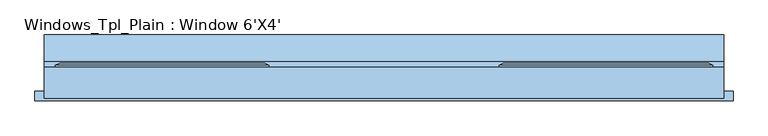
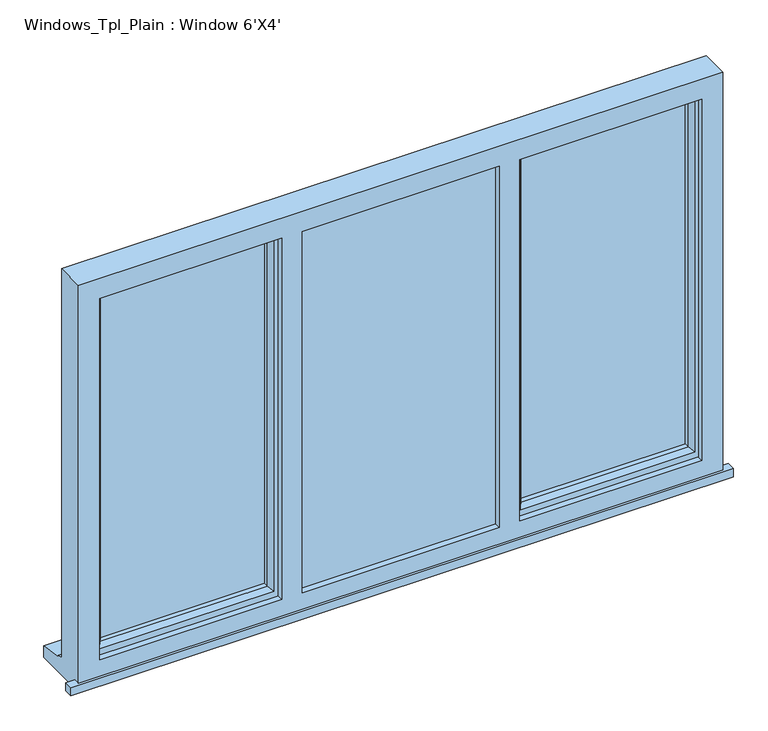
"""IFC4 building model written with IfcOpenShell, lengths in millimetres: window geometry, Windows_Tpl_Plain : Window 6'X4'."""

from ifc_helpers import new_model, si_unit, frame, origin, place, context, project, spatial, polyline, outline, extrude, faceted_brep, source, transform, mapped, element, save


def windows_tpl_plain_window_6_x4_c470b90d(model_context):
    return source(origin(), model_context, "Body", "SolidModel", [
        extrude(outline(polyline([(-1519.2, -73.6934322), (-1519.2, -48.6934322), (-1494.2, -48.6934322), (-1494.2, -67.3934322), (334.6, -67.3934322), (334.6, -48.6934322), (359.6, -48.6934322), (359.6, -73.6934322), (-1519.2, -73.6934322)])), frame((0.0, 0.0, 890.8), z_axis=(0.0, 0.0, 1.0), x_axis=(1.0, 0.0, 0.0)), (0.0, 0.0, 1.0), 25.0),
        faceted_brep([(-270.0, 15.6065678, 2080.0), (-270.0, 21.3800705, 2080.0), (-270.0, 21.3800705, 943.8), (-270.0, 15.6065678, 943.8), (-260.0, -49.3934322, 2070.0), (-260.0, 15.6065678, 2070.0), (-260.0, 15.6065678, 953.8), (-260.0, -49.3934322, 953.8), (-220.0, -34.9005323, 2030.0), (-230.1480377, -49.3934322, 2040.1480377), (-230.1480377, -49.3934322, 983.6519623), (-220.0, -34.9005323, 993.8), (-220.0, -20.3934322, 2030.0), (-220.0, -20.3934322, 993.8), (-230.0, 3.6065678, 2040.0), (-230.0, -20.3934322, 2040.0), (-230.0, -20.3934322, 983.8), (-230.0, 3.6065678, 983.8), (-220.0, 21.3800705, 2030.0), (-220.0, 3.6065678, 2030.0), (-220.0, 3.6065678, 993.8), (-220.0, 21.3800705, 993.8), (-237.4457548, 27.1535732, 2047.4457548), (-237.4457548, 27.1535732, 976.3542452), (-259.2153903, 27.1535732, 2069.2153903), (-259.2153903, 27.1535732, 954.5846097), (304.6, 21.3800705, 943.8), (304.6, 15.6065678, 943.8), (294.6, 15.6065678, 953.8), (294.6, -49.3934322, 953.8), (264.7480377, -49.3934322, 983.6519623), (254.6, -34.9005323, 993.8), (254.6, -20.3934322, 993.8), (264.6, -20.3934322, 983.8), (264.6, 3.6065678, 983.8), (254.6, 3.6065678, 993.8), (254.6, 21.3800705, 993.8), (272.0457548, 27.1535732, 976.3542452), (293.8153903, 27.1535732, 954.5846097), (304.6, 21.3800705, 2080.0), (304.6, 15.6065678, 2080.0), (294.6, 15.6065678, 2070.0), (294.6, -49.3934322, 2070.0), (264.7480377, -49.3934322, 2040.1480377), (254.6, -34.9005323, 2030.0), (254.6, -20.3934322, 2030.0), (264.6, -20.3934322, 2040.0), (264.6, 3.6065678, 2040.0), (254.6, 3.6065678, 2030.0), (254.6, 21.3800705, 2030.0), (272.0457548, 27.1535732, 2047.4457548), (293.8153903, 27.1535732, 2069.2153903)], [[[0, 1, 2, 3]], [[4, 5, 6, 7]], [[8, 9, 10, 11]], [[12, 8, 11, 13]], [[14, 15, 16, 17]], [[18, 19, 20, 21]], [[22, 18, 21, 23]], [[1, 24, 25, 2]], [[3, 2, 26, 27]], [[7, 6, 28, 29]], [[11, 10, 30, 31]], [[13, 11, 31, 32]], [[17, 16, 33, 34]], [[21, 20, 35, 36]], [[23, 21, 36, 37]], [[2, 25, 38, 26]], [[27, 26, 39, 40]], [[29, 28, 41, 42]], [[31, 30, 43, 44]], [[32, 31, 44, 45]], [[34, 33, 46, 47]], [[36, 35, 48, 49]], [[37, 36, 49, 50]], [[26, 38, 51, 39]], [[40, 39, 1, 0]], [[3, 27, 40, 0], [5, 41, 28, 6]], [[42, 41, 5, 4]], [[7, 29, 42, 4], [9, 43, 30, 10]], [[44, 43, 9, 8]], [[45, 44, 8, 12]], [[15, 46, 33, 16], [13, 32, 45, 12]], [[47, 46, 15, 14]], [[17, 34, 47, 14], [19, 48, 35, 20]], [[49, 48, 19, 18]], [[50, 49, 18, 22]], [[24, 51, 38, 25], [23, 37, 50, 22]], [[39, 51, 24, 1]]]),
        faceted_brep([(-889.6, 15.6065678, 2080.0), (-889.6, 21.3800705, 2080.0), (-1464.2, 21.3800705, 2080.0), (-1464.2, 15.6065678, 2080.0), (-899.6, -49.3934322, 2070.0), (-899.6, 15.6065678, 2070.0), (-1454.2, 15.6065678, 2070.0), (-1454.2, -49.3934322, 2070.0), (-939.6, -34.9005323, 2030.0), (-929.4519623, -49.3934322, 2040.1480377), (-1424.3480377, -49.3934322, 2040.1480377), (-1414.2, -34.9005323, 2030.0), (-939.6, -20.3934322, 2030.0), (-1414.2, -20.3934322, 2030.0), (-929.6, 3.6065678, 2040.0), (-929.6, -20.3934322, 2040.0), (-1424.2, -20.3934322, 2040.0), (-1424.2, 3.6065678, 2040.0), (-939.6, 21.3800705, 2030.0), (-939.6, 3.6065678, 2030.0), (-1414.2, 3.6065678, 2030.0), (-1414.2, 21.3800705, 2030.0), (-920.7854344, 27.1535732, 2048.8145656), (-1433.0145656, 27.1535732, 2048.8145656), (-901.2307806, 27.1535732, 2068.3692194), (-1452.5692194, 27.1535732, 2068.3692194), (-1464.2, 21.3800705, 943.8), (-1464.2, 15.6065678, 943.8), (-1454.2, 15.6065678, 953.8), (-1454.2, -49.3934322, 953.8), (-1424.3480377, -49.3934322, 983.6519623), (-1414.2, -34.9005323, 993.8), (-1414.2, -20.3934322, 993.8), (-1424.2, -20.3934322, 983.8), (-1424.2, 3.6065678, 983.8), (-1414.2, 3.6065678, 993.8), (-1414.2, 21.3800705, 993.8), (-1433.0145656, 27.1535732, 974.9854344), (-1452.5692194, 27.1535732, 955.4307806), (-889.6, 21.3800705, 943.8), (-889.6, 15.6065678, 943.8), (-899.6, 15.6065678, 953.8), (-899.6, -49.3934322, 953.8), (-929.4519623, -49.3934322, 983.6519623), (-939.6, -34.9005323, 993.8), (-939.6, -20.3934322, 993.8), (-929.6, -20.3934322, 983.8), (-929.6, 3.6065678, 983.8), (-939.6, 3.6065678, 993.8), (-939.6, 21.3800705, 993.8), (-920.7854344, 27.1535732, 974.9854344), (-901.2307806, 27.1535732, 955.4307806)], [[[0, 1, 2, 3]], [[4, 5, 6, 7]], [[8, 9, 10, 11]], [[12, 8, 11, 13]], [[14, 15, 16, 17]], [[18, 19, 20, 21]], [[22, 18, 21, 23]], [[1, 24, 25, 2]], [[3, 2, 26, 27]], [[7, 6, 28, 29]], [[11, 10, 30, 31]], [[13, 11, 31, 32]], [[17, 16, 33, 34]], [[21, 20, 35, 36]], [[23, 21, 36, 37]], [[2, 25, 38, 26]], [[27, 26, 39, 40]], [[0, 3, 27, 40], [41, 28, 6, 5]], [[29, 28, 41, 42]], [[4, 7, 29, 42], [43, 30, 10, 9]], [[31, 30, 43, 44]], [[32, 31, 44, 45]], [[46, 33, 16, 15], [12, 13, 32, 45]], [[34, 33, 46, 47]], [[14, 17, 34, 47], [48, 35, 20, 19]], [[36, 35, 48, 49]], [[37, 36, 49, 50]], [[51, 38, 25, 24], [22, 23, 37, 50]], [[26, 38, 51, 39]], [[40, 39, 1, 0]], [[42, 41, 5, 4]], [[44, 43, 9, 8]], [[45, 44, 8, 12]], [[47, 46, 15, 14]], [[49, 48, 19, 18]], [[50, 49, 18, 22]], [[39, 51, 24, 1]]]),
        faceted_brep([(334.6, -67.3934322, 2110.0), (-1494.2, -67.3934322, 2110.0), (-1494.2, -67.3934322, 890.8), (334.6, -67.3934322, 890.8), (274.6, -67.3934322, 2050.0), (274.6, -67.3934322, 965.8), (-242.0, -67.3934322, 965.8), (-242.0, -67.3934322, 2050.0), (-300.0, -67.3934322, 2050.0), (-300.0, -67.3934322, 965.8), (-859.6, -67.3934322, 965.8), (-859.6, -67.3934322, 2050.0), (-917.6, -67.3934322, 2050.0), (-917.6, -67.3934322, 965.8), (-1434.2, -67.3934322, 965.8), (-1434.2, -67.3934322, 2050.0), (-1494.2, 15.6065678, 2110.0), (-1494.2, 15.6065678, 941.8), (-1494.2, 30.6065678, 940.48767), (-1494.2, 30.6065678, 935.5449676), (-1494.2, 103.1065678, 924.6088847), (-1494.2, 103.1065678, 890.8), (334.6, 15.6065678, 2110.0), (334.6, 15.6065678, 941.8), (-1454.2, 15.6065678, 2070.0), (-1454.2, 15.6065678, 953.8), (-899.6, 15.6065678, 953.8), (-899.6, 15.6065678, 2070.0), (-859.6, 15.6065678, 2070.0), (-859.6, 15.6065678, 953.8), (-300.0, 15.6065678, 953.8), (-300.0, 15.6065678, 2070.0), (-260.0, 15.6065678, 2070.0), (-260.0, 15.6065678, 953.8), (294.6, 15.6065678, 953.8), (294.6, 15.6065678, 2070.0), (-1454.2, -49.3934322, 2070.0), (-1454.2, -49.3934322, 953.8), (-869.6, -49.3934322, 2070.0), (-290.0, -49.3934322, 2070.0), (-290.0, -49.3934322, 953.8), (-869.6, -49.3934322, 953.8), (-300.0, -49.3934322, 2050.0), (-859.6, -49.3934322, 2050.0), (-859.6, -49.3934322, 965.8), (-300.0, -49.3934322, 965.8), (-260.0, -49.3934322, 2070.0), (294.6, -49.3934322, 2070.0), (294.6, -49.3934322, 953.8), (-260.0, -49.3934322, 953.8), (274.6, -49.3934322, 2050.0), (-242.0, -49.3934322, 2050.0), (-242.0, -49.3934322, 965.8), (274.6, -49.3934322, 965.8), (-899.6, -49.3934322, 2070.0), (-899.6, -49.3934322, 953.8), (-917.6, -49.3934322, 2050.0), (-1434.2, -49.3934322, 2050.0), (-1434.2, -49.3934322, 965.8), (-917.6, -49.3934322, 965.8), (-859.6, -25.3934322, 2070.0), (-300.0, -25.3934322, 2070.0), (-290.0, -25.3934322, 2070.0), (-869.6, -25.3934322, 2070.0), (334.6, 103.1065678, 890.8), (334.6, 103.1065678, 924.6088847), (334.6, 30.6065678, 935.5449676), (334.6, 30.6065678, 940.48767), (-859.6, -25.3934322, 953.8), (-869.6, -25.3934322, 953.8), (-290.0, -25.3934322, 953.8), (-300.0, -25.3934322, 953.8)], [[[0, 1, 2, 3], [4, 5, 6, 7], [8, 9, 10, 11], [12, 13, 14, 15]], [[2, 1, 16, 17, 18, 19, 20, 21]], [[17, 16, 22, 23], [24, 25, 26, 27], [28, 29, 30, 31], [32, 33, 34, 35]], [[25, 24, 36, 37]], [[38, 39, 40, 41], [42, 43, 44, 45]], [[46, 47, 48, 49], [50, 51, 52, 53]], [[36, 54, 55, 37], [56, 57, 58, 59]], [[57, 15, 14, 58]], [[1, 0, 22, 16]], [[36, 24, 27, 54]], [[35, 47, 46, 32]], [[60, 28, 31, 61, 62, 39, 38, 63]], [[15, 57, 56, 12]], [[50, 4, 7, 51]], [[11, 43, 42, 8]], [[23, 22, 0, 3, 64, 65, 66, 67]], [[35, 34, 48, 47]], [[4, 50, 53, 5]], [[43, 11, 10, 44]], [[12, 56, 59, 13]], [[27, 26, 55, 54]], [[29, 28, 60, 68]], [[68, 60, 63, 69]], [[69, 63, 38, 41]], [[62, 70, 40, 39]], [[70, 62, 61, 71]], [[71, 61, 31, 30]], [[33, 32, 46, 49]], [[51, 7, 6, 52]], [[8, 42, 45, 9]], [[64, 3, 2, 21]], [[65, 64, 21, 20]], [[66, 65, 20, 19]], [[67, 66, 19, 18]], [[23, 67, 18, 17]], [[26, 25, 37, 55]], [[34, 33, 49, 48]], [[41, 40, 70, 71, 30, 29, 68, 69]], [[6, 5, 53, 52]], [[45, 44, 10, 9]], [[59, 58, 14, 13]]]),
        extrude(outline(polyline([(-929.6, -20.3934322), (-1424.2, -20.3934322), (-1424.2, 3.6065678), (-929.6, 3.6065678), (-929.6, -20.3934322)])), frame((0.0, 0.0, 983.8), z_axis=(0.0, 0.0, 1.0), x_axis=(1.0, 0.0, 0.0)), (0.0, 0.0, 1.0), 1056.2),
        extrude(outline(polyline([(-869.6, -25.3934322), (-290.0, -25.3934322), (-290.0, -49.3934322), (-869.6, -49.3934322), (-869.6, -25.3934322)])), frame((0.0, 0.0, 953.8), z_axis=(0.0, 0.0, 1.0), x_axis=(1.0, 0.0, 0.0)), (0.0, 0.0, 1.0), 1116.2),
        extrude(outline(polyline([(264.6, -20.3934322), (-230.0, -20.3934322), (-230.0, 3.6065678), (264.6, 3.6065678), (264.6, -20.3934322)])), frame((0.0, 0.0, 983.8), z_axis=(0.0, 0.0, 1.0), x_axis=(1.0, 0.0, 0.0)), (0.0, 0.0, 1.0), 1056.2),
    ])


if __name__ == "__main__":
    model = new_model("IFC4")
    model_context = context("Model", 3, world=origin())
    ifc_project = project(units=[si_unit("LENGTHUNIT", "METRE", prefix="MILLI")], contexts=[model_context])
    site = spatial("IfcSite", under=ifc_project)
    building = spatial("IfcBuilding", under=site)
    placement = place(None, origin())
    windows_tpl_plain_window_6_x4_shape = windows_tpl_plain_window_6_x4_c470b90d(model_context)
    element("IfcWindow", 1, ObjectType="Windows_Tpl_Plain : Window 6'X4'", at=placement, inside=building, context=model_context, shape_type="MappedRepresentation", body=[
        mapped(windows_tpl_plain_window_6_x4_shape, transform((0.0, 0.0, 0.0), x_axis=(1.0, 0.0, 0.0), y_axis=(0.0, 1.0, 0.0), z_axis=(0.0, 0.0, 1.0))),
    ])
    save(model, "model.ifc")

# Revit data of these elements
# Type "Windows_Tpl_Plain : Window 6'X4'"
#   Type Mark = "24"
#   Operation = "TriplePanelVertical"
#   Construction Type Id = "GSP4R"
#   Manufacturer = "Revit"
#   Keynote = "L10"
#   Analytic Construction = "1/8 in Pilkington single glazing"
#   Wrap Layers (Ext) from Ext = 0' - 4.03543"
#   Wrap Layers (Int) from Ext = 0' - 6.98819"
#   Window Board Projection = 0' - 0.98425"
#   Window Board Extension = 0' - 0.98425"
#   Visual Light Transmittance = 0.9
#   Solar Heat Gain Coefficient = 0.78
#   Rough Width = 6' - 0"
#   Rough Height = 4' - 0"
#   Height = 4' - 0"
#   Width = 6' - 0"
#   Heat Transfer Coefficient (U) = 0.6496 BTU/(h·ft²·°F)
#   Glazing Thickness = 0' - 0.94488"
#   FrameOffset - External = 0' - 1.9685"
#   Frame Depth = 0' - 2.55906"
#   Default Head Height = 6' - 11.07087"
#   Cill Depth = 0' - 3.44488"
#   Cavity Closer Width = 0' - 1.9685"
#   Cavity Closer Offset from Ext = 0' - 4.03543"
#   Cavity Closer Depth = 0' - 3.34646"
#   Vis - Cavity Closers = yes
#   Define Thermal Properties by = 1
#   Material Trim = Window Frame
#   Material Glass = Glass
#   Material Frame = Window Frame
#   Wall Closure = (empty or 0)
# Element 1 (IfcWindow, "Windows_Tpl_Plain : Window 6'X4'")
#   Materials on its faces: "Window Frame", "Glass"
# Materials
#   "Window Frame": colour RGB 249 249 249, transparency 0
#   "Glass": class "Glass", colour RGB 0 128 192, transparency 0.75, Description = "Soda Lime Glass", Cost = 0
